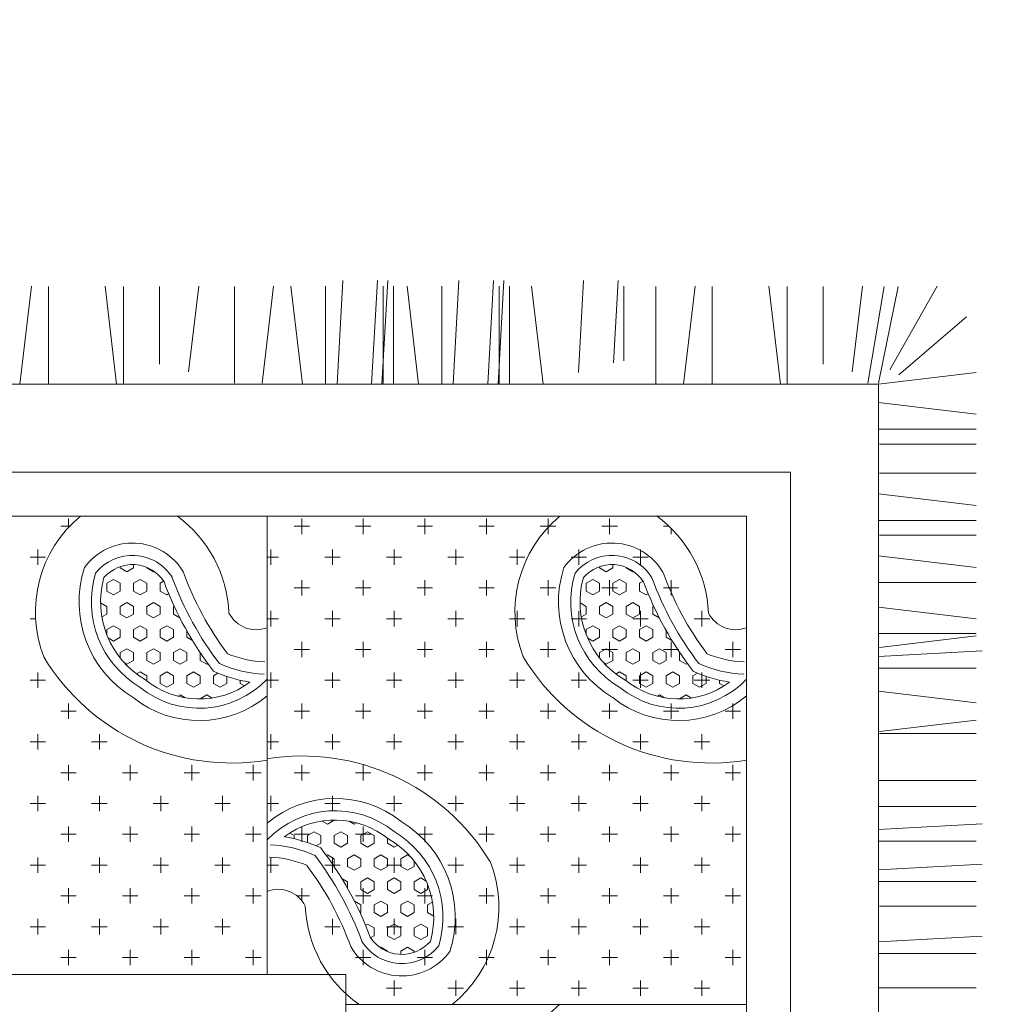
# Model space of a CAD drawing. Units: inches. Extents: x -638 to 186, y -762 to 59.
# Tile 10 of 31: x -117.58 to -100.41, y -474.18 to -456.78. Entities that reach past the tile are written whole.
import ezdxf

# ---------------------------------------------------------------- set-up
doc = ezdxf.new("R2010")
doc.units = ezdxf.units.IN
doc.layers.add('A-ANNO-DIMS', color=2, linetype='Continuous', lineweight=18)
doc.layers.add('furn', color=8, linetype='Continuous', lineweight=13)
doc.styles.get("Standard").update_dxf_attribs({"font": 'arial.ttf'})
doc.dimstyles.new('ISO-25', dxfattribs={"dimtxt": 4, "dimasz": 4, "dimexe": 1.25, "dimexo": 0.625, "dimtad": 0, "dimlunit": 4, "dimtxsty": 'Standard', "dimcen": 2.5, "dimclrt": 256, "dimadec": 0, "dimazin": 0, "dimtfac": 1, "dimtmove": 0, "dimatfit": 3, "dimfxl": 1, "dimfxlon": 1, "dimarcsym": 0})

# ---------------------------------------------------------------- blocks, each defined once
blk = doc.blocks.new('BED-DOUBLE-WITH-NIGHTSTANDS')
for p, q in [((58.548, 11.244), (58.548, 59.951)), ((68.982, 31.914), (68.982, 1.829)), ((67.427, 30.359), (67.427, 3.384)), ((66.65, 29.582), (66.65, 4.161)), ((68.982, 17.003), (70.71, 16.797)), ((59.394, 16.552), (59.394, 16.825)), ((60.483, 16.552), (60.483, 16.825)), ((61.571, 16.552), (61.571, 16.825)), ((62.659, 16.552), (62.659, 16.825)), ((63.748, 16.552), (63.748, 16.825)), ((64.836, 16.726), (64.836, 16.825)), ((65.924, 16.552), (65.924, 16.825)), ((59.258, 16.688), (59.53, 16.688)), ((60.346, 16.688), (60.619, 16.688)), ((61.435, 16.688), (61.707, 16.688)), ((62.523, 16.688), (62.795, 16.688)), ((63.612, 16.688), (63.884, 16.688)), ((65.788, 16.688), (66.06, 16.688)), ((68.982, 16.497), (70.707, 16.497)), ((58.85, 16.008), (58.85, 16.28)), ((59.938, 16.008), (59.938, 16.28)), ((61.027, 16.008), (61.027, 16.28)), ((62.115, 16.008), (62.115, 16.28)), ((63.203, 16.008), (63.203, 16.28)), ((66.468, 16.127), (66.468, 16.28)), ((58.714, 16.144), (58.986, 16.144)), ((59.802, 16.144), (60.074, 16.144)), ((60.891, 16.144), (61.163, 16.144)), ((61.979, 16.144), (62.251, 16.144)), ((63.067, 16.144), (63.339, 16.144)), ((66.45, 16.144), (66.605, 16.144)), ((59.394, 15.464), (59.394, 15.736)), ((60.483, 15.464), (60.483, 15.736)), ((61.571, 15.464), (61.571, 15.736)), ((62.659, 15.464), (62.659, 15.736)), ((59.258, 15.6), (59.53, 15.6)), ((60.346, 15.6), (60.619, 15.6)), ((61.435, 15.6), (61.707, 15.6)), ((62.523, 15.6), (62.795, 15.6)), ((64.917, 15.469), (64.866, 15.556)), ((65.053, 15.469), (65.116, 15.579)), ((68.982, 15.294), (70.71, 15.497)), ((64.44, 15.351), (64.495, 15.445)), ((64.508, 15.233), (64.44, 15.351)), ((64.552, 15.469), (64.644, 15.469)), ((64.712, 15.351), (64.644, 15.469)), ((64.644, 15.233), (64.712, 15.351)), ((64.917, 15.469), (65.053, 15.469)), ((65.257, 15.351), (65.325, 15.469)), ((65.325, 15.233), (65.257, 15.351)), ((65.325, 15.469), (65.461, 15.469)), ((65.529, 15.351), (65.461, 15.469)), ((65.461, 15.233), (65.529, 15.351)), ((58.85, 14.92), (58.85, 15.192)), ((59.938, 14.92), (59.938, 15.192)), ((61.027, 14.92), (61.027, 15.192)), ((62.115, 14.92), (62.115, 15.192)), ((64.032, 15.115), (64.059, 15.161)), ((64.143, 15.233), (64.236, 15.233)), ((64.304, 15.115), (64.236, 15.233)), ((64.508, 15.233), (64.644, 15.233)), ((64.849, 15.115), (64.917, 15.233)), ((64.917, 15.233), (65.053, 15.233)), ((65.121, 15.115), (65.053, 15.233)), ((65.325, 15.233), (65.461, 15.233)), ((65.665, 15.115), (65.733, 15.233)), ((65.733, 15.233), (65.755, 15.233)), ((68.982, 15.174), (70.707, 15.174)), ((58.714, 15.056), (58.986, 15.056)), ((59.802, 15.056), (60.074, 15.056)), ((60.891, 15.056), (61.163, 15.056)), ((61.979, 15.056), (62.251, 15.056)), ((64.1, 14.997), (64.032, 15.115)), ((64.1, 14.997), (64.236, 14.997)), ((64.236, 14.997), (64.304, 15.115)), ((64.44, 14.88), (64.508, 14.997)), ((64.508, 14.997), (64.644, 14.997)), ((64.712, 14.88), (64.644, 14.997)), ((64.917, 14.997), (64.849, 15.115)), ((64.917, 14.997), (65.053, 14.997)), ((65.053, 14.997), (65.121, 15.115)), ((65.257, 14.88), (65.325, 14.997)), ((65.325, 14.997), (65.461, 14.997)), ((65.529, 14.88), (65.461, 14.997)), ((65.733, 14.997), (65.665, 15.115)), ((65.733, 14.997), (65.791, 14.997)), ((63.828, 14.762), (63.896, 14.88)), ((63.896, 14.88), (63.86, 14.942)), ((64.508, 14.762), (64.44, 14.88)), ((64.644, 14.762), (64.712, 14.88)), ((65.325, 14.762), (65.257, 14.88)), ((65.461, 14.762), (65.529, 14.88)), ((59.394, 14.376), (59.394, 14.648)), ((60.483, 14.376), (60.483, 14.648)), ((61.571, 14.376), (61.571, 14.648)), ((63.737, 14.762), (63.828, 14.762)), ((64.032, 14.644), (64.1, 14.762)), ((64.1, 14.526), (64.032, 14.644)), ((64.1, 14.762), (64.236, 14.762)), ((64.304, 14.644), (64.236, 14.762)), ((64.236, 14.526), (64.304, 14.644)), ((64.508, 14.762), (64.644, 14.762)), ((64.849, 14.644), (64.917, 14.762)), ((64.917, 14.526), (64.849, 14.644)), ((64.917, 14.762), (65.053, 14.762)), ((65.121, 14.644), (65.053, 14.762)), ((65.053, 14.526), (65.121, 14.644)), ((65.325, 14.762), (65.461, 14.762)), ((65.665, 14.644), (65.733, 14.762)), ((65.671, 14.634), (65.665, 14.644)), ((65.733, 14.762), (65.741, 14.762)), ((59.258, 14.512), (59.53, 14.512)), ((60.346, 14.512), (60.619, 14.512)), ((61.435, 14.512), (61.707, 14.512)), ((63.624, 14.408), (63.692, 14.526)), ((63.692, 14.526), (63.828, 14.526)), ((63.896, 14.408), (63.828, 14.526)), ((64.1, 14.526), (64.236, 14.526)), ((64.44, 14.408), (64.508, 14.526)), ((64.508, 14.526), (64.644, 14.526)), ((64.712, 14.408), (64.644, 14.526)), ((64.917, 14.526), (65.053, 14.526)), ((65.257, 14.408), (65.325, 14.526)), ((65.325, 14.526), (65.461, 14.526)), ((65.497, 14.464), (65.461, 14.526)), ((69.331, 14.538), (70.707, 14.538)), ((63.692, 14.291), (63.624, 14.408)), ((63.692, 14.291), (63.828, 14.291)), ((63.828, 14.291), (63.896, 14.408)), ((64.032, 14.173), (64.1, 14.291)), ((64.1, 14.291), (64.236, 14.291)), ((64.304, 14.173), (64.236, 14.291)), ((64.508, 14.291), (64.44, 14.408)), ((64.508, 14.291), (64.644, 14.291)), ((64.644, 14.291), (64.712, 14.408)), ((64.852, 14.179), (64.917, 14.291)), ((64.917, 14.291), (65.053, 14.291)), ((65.059, 14.28), (65.053, 14.291)), ((65.276, 14.375), (65.257, 14.408)), ((58.85, 13.832), (58.85, 14.104)), ((59.938, 13.832), (59.938, 14.104)), ((61.027, 13.832), (61.027, 14.104)), ((62.115, 13.832), (62.115, 14.104)), ((63.438, 14.086), (63.488, 14.173)), ((63.488, 14.173), (63.465, 14.213)), ((64.1, 14.055), (64.032, 14.173)), ((64.236, 14.055), (64.304, 14.173)), ((58.714, 13.968), (58.986, 13.968)), ((59.802, 13.968), (60.074, 13.968)), ((60.891, 13.968), (61.163, 13.968)), ((61.979, 13.968), (62.251, 13.968)), ((63.624, 13.937), (63.692, 14.055)), ((63.692, 13.819), (63.624, 13.937)), ((63.692, 14.055), (63.828, 14.055)), ((63.896, 13.937), (63.828, 14.055)), ((63.828, 13.819), (63.896, 13.937)), ((64.1, 14.055), (64.236, 14.055)), ((64.451, 13.955), (64.508, 14.055)), ((64.508, 14.055), (64.621, 14.055)), ((69.195, 14.023), (70.71, 13.844)), ((63.417, 13.819), (63.42, 13.819)), ((63.488, 13.701), (63.42, 13.819)), ((63.692, 13.819), (63.828, 13.819)), ((64.032, 13.701), (64.1, 13.819)), ((64.1, 13.819), (64.236, 13.819)), ((64.237, 13.818), (64.236, 13.819)), ((63.434, 13.608), (63.488, 13.701)), ((63.624, 13.466), (63.692, 13.584)), ((63.692, 13.584), (63.828, 13.584)), ((63.874, 13.504), (63.828, 13.584)), ((64.043, 13.682), (64.032, 13.701)), ((59.258, 13.423), (59.53, 13.423)), ((59.394, 13.287), (59.394, 13.559)), ((60.346, 13.423), (60.619, 13.423)), ((60.483, 13.287), (60.483, 13.559)), ((61.435, 13.423), (61.707, 13.423)), ((61.571, 13.287), (61.571, 13.559)), ((63.692, 13.348), (63.624, 13.466)), ((63.692, 13.348), (63.815, 13.348)), ((63.648, 13.036), (63.692, 13.112)), ((63.692, 13.112), (63.748, 13.112)), ((68.996, 13.214), (70.707, 13.214)), ((58.714, 12.879), (58.986, 12.879)), ((58.85, 12.743), (58.85, 13.015)), ((59.802, 12.879), (60.074, 12.879)), ((59.938, 12.743), (59.938, 13.015)), ((60.891, 12.879), (61.163, 12.879)), ((61.027, 12.743), (61.027, 13.015)), ((61.979, 12.879), (62.251, 12.879)), ((62.115, 12.743), (62.115, 13.015)), ((68.996, 12.723), (70.71, 12.52)), ((66.65, 12.635), (58.548, 12.635)), ((58.548, 12.635), (66.65, 12.635)), ((60.346, 12.568), (60.619, 12.568)), ((60.483, 12.432), (60.483, 12.635)), ((61.435, 12.568), (61.707, 12.568)), ((61.571, 12.432), (61.571, 12.635)), ((62.523, 12.568), (62.795, 12.568)), ((62.523, 12.568), (62.795, 12.568)), ((62.659, 12.432), (62.659, 12.635)), ((62.659, 12.432), (62.659, 12.635)), ((63.612, 12.568), (63.884, 12.568)), ((63.612, 12.568), (63.884, 12.568)), ((63.748, 12.432), (63.748, 12.635)), ((63.748, 12.432), (63.748, 12.635)), ((64.7, 12.568), (64.972, 12.568)), ((64.7, 12.568), (64.972, 12.568)), ((64.836, 12.432), (64.836, 12.635)), ((64.836, 12.432), (64.836, 12.635)), ((65.788, 12.568), (66.06, 12.568)), ((65.788, 12.568), (66.06, 12.568)), ((65.924, 12.432), (65.924, 12.635)), ((65.924, 12.432), (65.924, 12.635)), ((66.65, 12.635), (66.65, 4.161)), ((61.047, 12.233), (61.003, 12.157)), ((68.982, 12.011), (70.71, 12.214)), ((59.857, 12.024), (60.074, 12.024)), ((59.938, 11.888), (59.938, 12.107)), ((60.891, 12.024), (61.163, 12.024)), ((61.003, 12.157), (60.948, 12.157)), ((61.027, 11.888), (61.027, 12.16)), ((61.979, 12.024), (62.251, 12.024)), ((62.115, 11.888), (62.115, 12.16)), ((63.067, 12.024), (63.339, 12.024)), ((63.067, 12.024), (63.339, 12.024)), ((63.203, 11.888), (63.203, 12.16)), ((63.203, 11.888), (63.203, 12.16)), ((64.156, 12.024), (64.428, 12.024)), ((64.156, 12.024), (64.428, 12.024)), ((64.292, 11.888), (64.292, 12.16)), ((64.292, 11.888), (64.292, 12.16)), ((65.244, 12.024), (65.516, 12.024)), ((65.244, 12.024), (65.516, 12.024)), ((65.38, 11.888), (65.38, 12.16)), ((65.38, 11.888), (65.38, 12.16)), ((66.332, 12.024), (66.605, 12.024)), ((66.332, 12.024), (66.605, 12.024)), ((66.468, 11.888), (66.468, 12.16)), ((66.468, 11.888), (66.468, 12.16)), ((61.003, 11.921), (60.881, 11.921)), ((61.003, 11.921), (61.072, 11.804)), ((60.821, 11.766), (60.867, 11.686)), ((61.003, 11.686), (60.867, 11.686)), ((61.072, 11.804), (61.003, 11.686)), ((61.261, 11.661), (61.208, 11.568)), ((59.394, 11.344), (59.394, 11.616)), ((60.483, 11.344), (60.483, 11.616)), ((60.663, 11.568), (60.595, 11.45)), ((60.652, 11.587), (60.663, 11.568)), ((61.208, 11.568), (61.276, 11.45)), ((61.571, 11.344), (61.571, 11.616)), ((62.659, 11.344), (62.659, 11.616)), ((62.659, 11.344), (62.659, 11.616)), ((63.748, 11.344), (63.748, 11.616)), ((63.748, 11.344), (63.748, 11.616)), ((64.836, 11.344), (64.836, 11.616)), ((64.836, 11.344), (64.836, 11.616)), ((65.924, 11.344), (65.924, 11.616)), ((65.924, 11.344), (65.924, 11.616)), ((68.982, 11.603), (70.71, 11.603)), ((59.258, 11.48), (59.53, 11.48)), ((60.245, 11.315), (60.187, 11.215)), ((60.346, 11.48), (60.619, 11.48)), ((60.459, 11.451), (60.459, 11.45)), ((60.595, 11.45), (60.459, 11.45)), ((60.867, 11.45), (60.799, 11.332)), ((60.799, 11.332), (60.867, 11.215)), ((61.003, 11.45), (60.867, 11.45)), ((61.003, 11.45), (61.072, 11.332)), ((61.072, 11.332), (61.003, 11.215)), ((61.279, 11.45), (61.276, 11.45)), ((61.435, 11.48), (61.707, 11.48)), ((62.523, 11.48), (62.795, 11.48)), ((62.523, 11.48), (62.795, 11.48)), ((63.612, 11.48), (63.884, 11.48)), ((63.612, 11.48), (63.884, 11.48)), ((64.7, 11.48), (64.972, 11.48)), ((64.7, 11.48), (64.972, 11.48)), ((65.788, 11.48), (66.06, 11.48)), ((65.788, 11.48), (66.06, 11.48)), ((68.982, 11.4), (70.811, 11.298)), ((20.158, 11.244), (58.548, 11.244)), ((58.022, 4.161), (58.022, 11.244)), ((58.022, 11.244), (58.022, 4.161)), ((60.187, 11.215), (60.075, 11.215)), ((60.459, 11.215), (60.391, 11.097)), ((60.595, 11.215), (60.459, 11.215)), ((60.595, 11.215), (60.663, 11.097)), ((61.003, 11.215), (60.867, 11.215)), ((61.258, 11.184), (61.208, 11.097)), ((58.85, 10.8), (58.85, 11.072)), ((59.637, 10.99), (59.643, 10.979)), ((59.779, 10.979), (59.643, 10.979)), ((59.843, 11.09), (59.779, 10.979)), ((59.938, 10.8), (59.938, 11.072)), ((60.051, 10.979), (59.983, 10.861)), ((60.187, 10.979), (60.051, 10.979)), ((60.187, 10.979), (60.255, 10.861)), ((60.391, 11.097), (60.459, 10.979)), ((60.595, 10.979), (60.459, 10.979)), ((60.663, 11.097), (60.595, 10.979)), ((60.867, 10.979), (60.799, 10.861)), ((61.003, 10.979), (60.867, 10.979)), ((61.003, 10.979), (61.072, 10.861)), ((61.027, 10.8), (61.027, 11.072)), ((61.208, 11.097), (61.231, 11.057)), ((62.115, 10.8), (62.115, 11.072)), ((63.203, 10.8), (63.203, 11.072)), ((63.203, 10.8), (63.203, 11.072)), ((64.292, 10.8), (64.292, 11.072)), ((64.292, 10.8), (64.292, 11.072)), ((65.38, 10.8), (65.38, 11.072)), ((65.38, 10.8), (65.38, 11.072)), ((66.468, 10.8), (66.468, 11.072)), ((66.468, 10.8), (66.468, 11.072)), ((58.714, 10.936), (58.986, 10.936)), ((59.199, 10.806), (59.235, 10.743)), ((59.439, 10.861), (59.371, 10.743)), ((59.419, 10.895), (59.439, 10.861)), ((59.802, 10.936), (60.074, 10.936)), ((59.983, 10.861), (60.051, 10.743)), ((60.255, 10.861), (60.187, 10.743)), ((60.799, 10.861), (60.867, 10.743)), ((60.891, 10.936), (61.163, 10.936)), ((61.072, 10.861), (61.003, 10.743)), ((61.979, 10.936), (62.251, 10.936)), ((63.067, 10.936), (63.339, 10.936)), ((63.067, 10.936), (63.339, 10.936)), ((64.156, 10.936), (64.428, 10.936)), ((64.156, 10.936), (64.428, 10.936)), ((65.244, 10.936), (65.516, 10.936)), ((65.244, 10.936), (65.516, 10.936)), ((66.332, 10.936), (66.605, 10.936)), ((66.332, 10.936), (66.605, 10.936)), ((68.982, 10.789), (70.811, 10.687)), ((59.031, 10.625), (58.963, 10.508)), ((59.025, 10.636), (59.031, 10.625)), ((59.371, 10.743), (59.235, 10.743)), ((59.643, 10.743), (59.575, 10.625)), ((59.575, 10.625), (59.643, 10.508)), ((59.779, 10.743), (59.643, 10.743)), ((59.779, 10.743), (59.847, 10.625)), ((59.847, 10.625), (59.779, 10.508)), ((60.187, 10.743), (60.051, 10.743)), ((60.459, 10.743), (60.391, 10.625)), ((60.391, 10.625), (60.459, 10.508)), ((60.595, 10.743), (60.459, 10.743)), ((60.595, 10.743), (60.663, 10.625)), ((60.663, 10.625), (60.595, 10.508)), ((61.003, 10.743), (60.867, 10.743)), ((58.306, 10.256), (58.306, 10.528)), ((58.963, 10.508), (58.955, 10.508)), ((59.235, 10.508), (59.167, 10.39)), ((59.371, 10.508), (59.235, 10.508)), ((59.371, 10.508), (59.439, 10.39)), ((59.394, 10.256), (59.394, 10.528)), ((59.779, 10.508), (59.643, 10.508)), ((60.051, 10.508), (59.983, 10.39)), ((60.187, 10.508), (60.051, 10.508)), ((60.187, 10.508), (60.255, 10.39)), ((60.595, 10.508), (60.459, 10.508)), ((60.483, 10.256), (60.483, 10.528)), ((60.867, 10.508), (60.799, 10.39)), ((60.958, 10.508), (60.867, 10.508)), ((61.571, 10.256), (61.571, 10.528)), ((62.659, 10.256), (62.659, 10.528)), ((62.659, 10.256), (62.659, 10.528)), ((63.748, 10.256), (63.748, 10.528)), ((63.748, 10.256), (63.748, 10.528)), ((64.836, 10.256), (64.836, 10.528)), ((64.836, 10.256), (64.836, 10.528)), ((65.924, 10.256), (65.924, 10.528)), ((65.924, 10.256), (65.924, 10.528)), ((68.982, 10.606), (70.811, 10.504)), ((68.982, 10.585), (70.71, 10.585)), ((58.17, 10.392), (58.442, 10.392)), ((58.963, 10.272), (58.904, 10.272)), ((58.963, 10.272), (59.031, 10.154)), ((59.167, 10.39), (59.235, 10.272)), ((59.371, 10.272), (59.235, 10.272)), ((59.258, 10.392), (59.53, 10.392)), ((59.439, 10.39), (59.371, 10.272)), ((59.643, 10.272), (59.575, 10.154)), ((59.779, 10.272), (59.643, 10.272)), ((59.779, 10.272), (59.847, 10.154)), ((59.983, 10.39), (60.051, 10.272)), ((60.187, 10.272), (60.051, 10.272)), ((60.255, 10.39), (60.187, 10.272)), ((60.346, 10.392), (60.619, 10.392)), ((60.459, 10.272), (60.391, 10.154)), ((60.595, 10.272), (60.459, 10.272)), ((60.595, 10.272), (60.663, 10.154)), ((60.799, 10.39), (60.836, 10.327)), ((61.435, 10.392), (61.707, 10.392)), ((62.523, 10.392), (62.795, 10.392)), ((62.523, 10.392), (62.795, 10.392)), ((63.612, 10.392), (63.884, 10.392)), ((63.612, 10.392), (63.884, 10.392)), ((64.7, 10.392), (64.972, 10.392)), ((64.7, 10.392), (64.972, 10.392)), ((65.788, 10.392), (66.06, 10.392)), ((65.788, 10.392), (66.06, 10.392)), ((68.982, 10.402), (70.71, 10.402)), ((59.031, 10.154), (58.963, 10.036)), ((59.575, 10.154), (59.643, 10.036)), ((59.847, 10.154), (59.779, 10.036)), ((60.391, 10.154), (60.459, 10.036)), ((60.663, 10.154), (60.637, 10.108)), ((68.982, 9.957), (70.71, 10.161)), ((58.85, 9.711), (58.85, 9.983)), ((58.963, 10.036), (58.94, 10.036)), ((59.235, 10.036), (59.167, 9.919)), ((59.167, 9.919), (59.235, 9.801)), ((59.371, 10.036), (59.235, 10.036)), ((59.371, 10.036), (59.439, 9.919)), ((59.439, 9.919), (59.371, 9.801)), ((59.779, 10.036), (59.643, 10.036)), ((59.938, 9.711), (59.938, 9.983)), ((60.051, 10.036), (59.983, 9.919)), ((59.983, 9.919), (60.051, 9.801)), ((60.187, 10.036), (60.051, 10.036)), ((60.187, 10.036), (60.255, 9.919)), ((60.255, 9.919), (60.201, 9.825)), ((60.553, 10.036), (60.459, 10.036)), ((61.027, 9.711), (61.027, 9.983)), ((62.115, 9.711), (62.115, 9.983)), ((62.115, 9.711), (62.115, 9.983)), ((63.203, 9.711), (63.203, 9.983)), ((63.203, 9.711), (63.203, 9.983)), ((64.292, 9.711), (64.292, 9.983)), ((64.292, 9.711), (64.292, 9.983)), ((65.38, 9.711), (65.38, 9.983)), ((65.38, 9.711), (65.38, 9.983)), ((66.468, 9.711), (66.468, 9.983)), ((66.468, 9.711), (66.468, 9.983)), ((58.714, 9.847), (58.986, 9.847)), ((59.371, 9.801), (59.235, 9.801)), ((59.643, 9.801), (59.58, 9.691)), ((59.779, 9.801), (59.643, 9.801)), ((59.779, 9.801), (59.83, 9.713)), ((59.802, 9.847), (60.074, 9.847)), ((60.144, 9.801), (60.051, 9.801)), ((60.891, 9.847), (61.163, 9.847)), ((61.979, 9.847), (62.251, 9.847)), ((61.979, 9.847), (62.251, 9.847)), ((63.067, 9.847), (63.339, 9.847)), ((63.067, 9.847), (63.339, 9.847)), ((64.156, 9.847), (64.428, 9.847)), ((64.156, 9.847), (64.428, 9.847)), ((65.244, 9.847), (65.516, 9.847)), ((65.244, 9.847), (65.516, 9.847)), ((66.332, 9.847), (66.605, 9.847)), ((66.332, 9.847), (66.605, 9.847)), ((58.306, 9.167), (58.306, 9.439)), ((59.394, 9.167), (59.394, 9.439)), ((60.483, 9.167), (60.483, 9.439)), ((61.571, 9.167), (61.571, 9.439)), ((61.571, 9.167), (61.571, 9.439)), ((62.659, 9.167), (62.659, 9.439)), ((62.659, 9.167), (62.659, 9.439)), ((63.748, 9.167), (63.748, 9.439)), ((63.748, 9.167), (63.748, 9.439)), ((64.836, 9.167), (64.836, 9.439)), ((64.836, 9.167), (64.836, 9.439)), ((65.924, 9.167), (65.924, 9.439)), ((65.924, 9.167), (65.924, 9.439)), ((68.982, 9.55), (70.71, 9.55)), ((58.17, 9.303), (58.442, 9.303)), ((59.258, 9.303), (59.53, 9.303)), ((60.346, 9.303), (60.619, 9.303)), ((61.435, 9.303), (61.707, 9.303)), ((61.435, 9.303), (61.707, 9.303)), ((62.523, 9.303), (62.795, 9.303)), ((62.523, 9.303), (62.795, 9.303)), ((63.612, 9.303), (63.884, 9.303)), ((63.612, 9.303), (63.884, 9.303)), ((64.7, 9.303), (64.972, 9.303)), ((64.7, 9.303), (64.972, 9.303)), ((65.788, 9.303), (66.06, 9.303)), ((65.788, 9.303), (66.06, 9.303)), ((68.982, 9.347), (70.811, 9.245)), ((58.85, 8.623), (58.85, 8.895)), ((59.938, 8.623), (59.938, 8.895)), ((61.027, 8.623), (61.027, 8.895)), ((61.027, 8.623), (61.027, 8.895)), ((62.115, 8.623), (62.115, 8.895)), ((62.115, 8.623), (62.115, 8.895)), ((63.203, 8.623), (63.203, 8.895)), ((63.203, 8.623), (63.203, 8.895)), ((64.292, 8.623), (64.292, 8.895)), ((64.292, 8.623), (64.292, 8.895)), ((65.38, 8.623), (65.38, 8.895)), ((65.38, 8.623), (65.38, 8.895)), ((66.468, 8.623), (66.468, 8.895)), ((66.468, 8.623), (66.468, 8.895)), ((58.714, 8.759), (58.783, 8.759)), ((58.714, 8.759), (58.986, 8.759)), ((58.85, 8.623), (58.85, 8.728)), ((59.802, 8.759), (60.074, 8.759)), ((60.891, 8.759), (61.163, 8.759)), ((60.891, 8.759), (61.163, 8.759)), ((61.979, 8.759), (62.251, 8.759)), ((61.979, 8.759), (62.251, 8.759)), ((63.067, 8.759), (63.339, 8.759)), ((63.067, 8.759), (63.339, 8.759)), ((64.156, 8.759), (64.428, 8.759)), ((64.156, 8.759), (64.428, 8.759)), ((65.244, 8.759), (65.516, 8.759)), ((65.244, 8.759), (65.516, 8.759)), ((66.332, 8.759), (66.605, 8.759)), ((66.332, 8.759), (66.605, 8.759)), ((68.982, 8.736), (70.811, 8.634)), ((68.982, 8.553), (70.811, 8.451)), ((68.982, 8.532), (70.71, 8.532)), ((58.306, 8.079), (58.306, 8.351)), ((58.306, 8.079), (58.306, 8.351)), ((59.394, 8.079), (59.394, 8.351)), ((59.394, 8.079), (59.394, 8.351)), ((60.483, 8.079), (60.483, 8.351)), ((60.483, 8.079), (60.483, 8.351)), ((61.571, 8.079), (61.571, 8.351)), ((61.571, 8.079), (61.571, 8.351)), ((62.659, 8.079), (62.659, 8.351)), ((62.659, 8.079), (62.659, 8.351)), ((63.748, 8.079), (63.748, 8.351)), ((63.748, 8.079), (63.748, 8.351)), ((64.836, 8.253), (64.836, 8.351)), ((64.836, 8.079), (64.836, 8.351)), ((65.924, 8.079), (65.924, 8.351)), ((65.924, 8.079), (65.924, 8.351)), ((58.17, 8.215), (58.442, 8.215)), ((58.17, 8.215), (58.442, 8.215)), ((59.258, 8.215), (59.53, 8.215)), ((59.258, 8.215), (59.53, 8.215)), ((60.346, 8.215), (60.619, 8.215)), ((60.346, 8.215), (60.619, 8.215)), ((61.435, 8.215), (61.707, 8.215)), ((61.435, 8.215), (61.707, 8.215)), ((62.523, 8.215), (62.795, 8.215)), ((62.523, 8.215), (62.795, 8.215)), ((63.612, 8.215), (63.884, 8.215)), ((63.612, 8.215), (63.884, 8.215)), ((64.7, 8.215), (64.972, 8.215)), ((65.788, 8.215), (66.06, 8.215)), ((65.788, 8.215), (66.06, 8.215)), ((68.982, 8.349), (70.71, 8.349)), ((68.982, 7.757), (70.71, 7.961)), ((58.714, 7.671), (58.986, 7.671)), ((58.714, 7.671), (58.986, 7.671)), ((58.85, 7.535), (58.85, 7.807)), ((58.85, 7.535), (58.85, 7.807)), ((59.802, 7.671), (60.074, 7.671)), ((59.802, 7.671), (60.074, 7.671)), ((59.938, 7.535), (59.938, 7.807)), ((59.938, 7.535), (59.938, 7.807)), ((60.891, 7.671), (61.163, 7.671)), ((60.891, 7.671), (61.163, 7.671)), ((61.027, 7.535), (61.027, 7.807)), ((61.027, 7.535), (61.027, 7.807)), ((61.979, 7.671), (62.251, 7.671)), ((61.979, 7.671), (62.251, 7.671)), ((62.115, 7.535), (62.115, 7.807)), ((62.115, 7.535), (62.115, 7.807)), ((63.067, 7.671), (63.339, 7.671)), ((63.067, 7.671), (63.339, 7.671)), ((63.203, 7.535), (63.203, 7.807)), ((63.203, 7.535), (63.203, 7.807)), ((64.156, 7.671), (64.428, 7.671)), ((64.292, 7.535), (64.292, 7.807)), ((65.244, 7.671), (65.516, 7.671)), ((65.38, 7.535), (65.38, 7.807)), ((66.332, 7.671), (66.605, 7.671)), ((66.45, 7.671), (66.605, 7.671)), ((66.468, 7.653), (66.468, 7.807)), ((66.468, 7.535), (66.468, 7.807)), ((58.306, 6.99), (58.306, 7.263)), ((58.306, 6.99), (58.306, 7.263)), ((59.394, 6.99), (59.394, 7.263)), ((59.394, 6.99), (59.394, 7.263)), ((60.483, 6.99), (60.483, 7.263)), ((60.483, 6.99), (60.483, 7.263)), ((61.571, 6.99), (61.571, 7.263)), ((61.571, 6.99), (61.571, 7.263)), ((62.659, 6.99), (62.659, 7.263)), ((62.659, 6.99), (62.659, 7.263)), ((63.748, 6.99), (63.748, 7.263)), ((64.836, 6.99), (64.836, 7.263)), ((65.924, 6.99), (65.924, 7.263)), ((69.184, 7.135), (70.811, 7.044)), ((58.17, 7.127), (58.442, 7.127)), ((58.17, 7.127), (58.442, 7.127)), ((59.258, 7.127), (59.53, 7.127)), ((59.258, 7.127), (59.53, 7.127)), ((60.346, 7.127), (60.619, 7.127)), ((60.346, 7.127), (60.619, 7.127)), ((61.435, 7.127), (61.707, 7.127)), ((61.435, 7.127), (61.707, 7.127)), ((62.523, 7.127), (62.795, 7.127)), ((62.523, 7.127), (62.795, 7.127)), ((63.612, 7.127), (63.884, 7.127)), ((64.44, 6.877), (64.495, 6.971)), ((64.552, 6.995), (64.644, 6.995)), ((64.712, 6.877), (64.644, 6.995)), ((64.7, 7.127), (64.972, 7.127)), ((64.917, 6.995), (64.866, 7.082)), ((64.917, 6.995), (65.053, 6.995)), ((65.053, 6.995), (65.116, 7.105)), ((65.257, 6.877), (65.325, 6.995)), ((65.325, 6.995), (65.461, 6.995)), ((65.529, 6.877), (65.461, 6.995)), ((65.788, 7.127), (66.06, 7.127)), ((64.508, 6.76), (64.44, 6.877)), ((64.644, 6.76), (64.712, 6.877)), ((65.325, 6.76), (65.257, 6.877)), ((65.461, 6.76), (65.529, 6.877)), ((58.85, 6.446), (58.85, 6.718)), ((58.85, 6.446), (58.85, 6.718)), ((59.938, 6.446), (59.938, 6.718)), ((59.938, 6.446), (59.938, 6.718)), ((61.027, 6.446), (61.027, 6.718)), ((61.027, 6.446), (61.027, 6.718)), ((62.115, 6.446), (62.115, 6.718)), ((62.115, 6.446), (62.115, 6.718)), ((63.203, 6.446), (63.203, 6.718)), ((64.032, 6.642), (64.059, 6.688)), ((64.1, 6.524), (64.032, 6.642)), ((64.143, 6.76), (64.236, 6.76)), ((64.304, 6.642), (64.236, 6.76)), ((64.236, 6.524), (64.304, 6.642)), ((64.292, 6.446), (64.292, 6.718)), ((64.508, 6.76), (64.644, 6.76)), ((64.849, 6.642), (64.917, 6.76)), ((64.917, 6.524), (64.849, 6.642)), ((64.917, 6.76), (65.053, 6.76)), ((65.121, 6.642), (65.053, 6.76)), ((65.053, 6.524), (65.121, 6.642)), ((65.325, 6.76), (65.461, 6.76)), ((65.38, 6.446), (65.38, 6.718)), ((65.665, 6.642), (65.733, 6.76)), ((65.733, 6.524), (65.665, 6.642)), ((65.733, 6.76), (65.755, 6.76)), ((66.468, 6.446), (66.468, 6.718)), ((58.714, 6.582), (58.986, 6.582)), ((58.714, 6.582), (58.986, 6.582)), ((59.802, 6.582), (60.074, 6.582)), ((59.802, 6.582), (60.074, 6.582)), ((60.891, 6.582), (61.163, 6.582)), ((60.891, 6.582), (61.163, 6.582)), ((61.979, 6.582), (62.251, 6.582)), ((61.979, 6.582), (62.251, 6.582)), ((63.067, 6.582), (63.339, 6.582)), ((63.896, 6.406), (63.86, 6.469)), ((64.1, 6.524), (64.236, 6.524)), ((64.156, 6.582), (64.428, 6.582)), ((64.44, 6.406), (64.508, 6.524)), ((64.508, 6.524), (64.644, 6.524)), ((64.712, 6.406), (64.644, 6.524)), ((64.917, 6.524), (65.053, 6.524)), ((65.244, 6.582), (65.516, 6.582)), ((65.257, 6.406), (65.325, 6.524)), ((65.325, 6.524), (65.461, 6.524)), ((65.529, 6.406), (65.461, 6.524)), ((65.733, 6.524), (65.791, 6.524)), ((66.332, 6.582), (66.605, 6.582)), ((69.357, 6.514), (70.811, 6.433)), ((63.737, 6.288), (63.828, 6.288)), ((63.828, 6.288), (63.896, 6.406)), ((64.032, 6.17), (64.1, 6.288)), ((64.1, 6.288), (64.236, 6.288)), ((64.304, 6.17), (64.236, 6.288)), ((64.508, 6.288), (64.44, 6.406)), ((64.508, 6.288), (64.644, 6.288)), ((64.644, 6.288), (64.712, 6.406)), ((64.849, 6.17), (64.917, 6.288)), ((64.917, 6.288), (65.053, 6.288)), ((65.121, 6.17), (65.053, 6.288)), ((65.325, 6.288), (65.257, 6.406)), ((65.325, 6.288), (65.461, 6.288)), ((65.461, 6.288), (65.529, 6.406)), ((65.665, 6.17), (65.733, 6.288)), ((65.733, 6.288), (65.741, 6.288)), ((69.393, 6.332), (70.71, 6.332)), ((58.306, 5.902), (58.306, 6.174)), ((58.306, 5.902), (58.306, 6.174)), ((59.394, 5.902), (59.394, 6.174)), ((59.394, 5.902), (59.394, 6.174)), ((60.483, 5.902), (60.483, 6.174)), ((60.483, 5.902), (60.483, 6.174)), ((61.571, 5.902), (61.571, 6.174)), ((61.571, 5.902), (61.571, 6.174)), ((62.659, 5.902), (62.659, 6.174)), ((63.748, 5.902), (63.748, 6.174)), ((64.1, 6.053), (64.032, 6.17)), ((64.236, 6.053), (64.304, 6.17)), ((64.836, 5.902), (64.836, 6.174)), ((64.917, 6.053), (64.849, 6.17)), ((65.053, 6.053), (65.121, 6.17)), ((65.671, 6.16), (65.665, 6.17)), ((65.924, 5.902), (65.924, 6.174)), ((58.17, 6.038), (58.442, 6.038)), ((58.17, 6.038), (58.442, 6.038)), ((59.258, 6.038), (59.53, 6.038)), ((59.258, 6.038), (59.53, 6.038)), ((60.346, 6.038), (60.619, 6.038)), ((60.346, 6.038), (60.619, 6.038)), ((61.435, 6.038), (61.707, 6.038)), ((61.435, 6.038), (61.707, 6.038)), ((62.523, 6.038), (62.795, 6.038)), ((63.612, 6.038), (63.884, 6.038)), ((63.624, 5.935), (63.692, 6.053)), ((63.692, 5.817), (63.624, 5.935)), ((63.692, 6.053), (63.828, 6.053)), ((63.896, 5.935), (63.828, 6.053)), ((63.828, 5.817), (63.896, 5.935)), ((64.1, 6.053), (64.236, 6.053)), ((64.44, 5.935), (64.508, 6.053)), ((64.508, 5.817), (64.44, 5.935)), ((64.508, 6.053), (64.644, 6.053)), ((64.712, 5.935), (64.644, 6.053)), ((64.644, 5.817), (64.712, 5.935)), ((64.7, 6.038), (64.972, 6.038)), ((64.917, 6.053), (65.053, 6.053)), ((65.257, 5.935), (65.325, 6.053)), ((65.276, 5.901), (65.257, 5.935)), ((65.325, 6.053), (65.461, 6.053)), ((65.497, 5.99), (65.461, 6.053)), ((65.788, 6.038), (66.06, 6.038)), ((63.692, 5.817), (63.828, 5.817)), ((64.032, 5.699), (64.1, 5.817)), ((64.1, 5.817), (64.236, 5.817)), ((64.304, 5.699), (64.236, 5.817)), ((64.508, 5.817), (64.644, 5.817)), ((64.852, 5.706), (64.917, 5.817)), ((64.917, 5.817), (65.053, 5.817)), ((65.059, 5.806), (65.053, 5.817)), ((68.982, 5.764), (70.707, 5.764)), ((58.85, 5.358), (58.85, 5.63)), ((58.85, 5.358), (58.85, 5.63)), ((59.938, 5.358), (59.938, 5.63)), ((59.938, 5.358), (59.938, 5.63)), ((61.027, 5.358), (61.027, 5.63)), ((61.027, 5.358), (61.027, 5.63)), ((62.115, 5.358), (62.115, 5.63)), ((62.115, 5.358), (62.115, 5.63)), ((63.203, 5.358), (63.203, 5.63)), ((63.438, 5.612), (63.488, 5.699)), ((63.488, 5.699), (63.465, 5.739)), ((63.624, 5.464), (63.692, 5.581)), ((63.692, 5.581), (63.828, 5.581)), ((63.896, 5.464), (63.828, 5.581)), ((64.1, 5.581), (64.032, 5.699)), ((64.1, 5.581), (64.236, 5.581)), ((64.236, 5.581), (64.304, 5.699)), ((64.292, 5.358), (64.292, 5.63)), ((64.451, 5.481), (64.508, 5.581)), ((64.508, 5.581), (64.621, 5.581)), ((65.38, 5.358), (65.38, 5.63)), ((66.468, 5.533), (66.468, 5.63)), ((58.714, 5.494), (58.986, 5.494)), ((58.714, 5.494), (58.986, 5.494)), ((59.802, 5.494), (60.074, 5.494)), ((59.802, 5.494), (60.074, 5.494)), ((60.891, 5.494), (61.163, 5.494)), ((60.891, 5.494), (61.163, 5.494)), ((61.979, 5.494), (62.251, 5.494)), ((61.979, 5.494), (62.251, 5.494)), ((63.067, 5.494), (63.339, 5.494)), ((63.692, 5.346), (63.624, 5.464)), ((63.828, 5.346), (63.896, 5.464)), ((64.156, 5.494), (64.428, 5.494)), ((65.244, 5.494), (65.516, 5.494)), ((66.332, 5.494), (66.43, 5.494)), ((63.417, 5.346), (63.42, 5.346)), ((63.488, 5.228), (63.42, 5.346)), ((63.434, 5.135), (63.488, 5.228)), ((63.692, 5.346), (63.828, 5.346)), ((64.032, 5.228), (64.1, 5.346)), ((64.043, 5.209), (64.032, 5.228)), ((64.1, 5.346), (64.236, 5.346)), ((64.237, 5.344), (64.236, 5.346)), ((68.982, 5.274), (70.71, 5.069)), ((58.306, 4.814), (58.306, 5.086)), ((58.306, 4.814), (58.306, 5.086)), ((59.394, 4.814), (59.394, 5.086)), ((59.394, 4.814), (59.394, 5.086)), ((60.483, 4.814), (60.483, 5.086)), ((60.483, 4.814), (60.483, 5.086)), ((61.571, 4.814), (61.571, 5.086)), ((61.571, 4.814), (61.571, 5.086)), ((62.659, 4.814), (62.659, 5.086)), ((63.624, 4.992), (63.692, 5.11)), ((63.692, 5.11), (63.828, 5.11)), ((63.748, 4.814), (63.748, 5.086)), ((63.874, 5.03), (63.828, 5.11)), ((64.836, 4.814), (64.836, 5.086)), ((58.17, 4.95), (58.442, 4.95)), ((58.17, 4.95), (58.442, 4.95)), ((59.258, 4.95), (59.53, 4.95)), ((59.258, 4.95), (59.53, 4.95)), ((60.346, 4.95), (60.619, 4.95)), ((60.346, 4.95), (60.619, 4.95)), ((61.435, 4.95), (61.707, 4.95)), ((61.435, 4.95), (61.707, 4.95)), ((62.523, 4.95), (62.795, 4.95)), ((63.612, 4.95), (63.884, 4.95)), ((63.692, 4.874), (63.624, 4.992)), ((63.692, 4.874), (63.815, 4.874)), ((64.7, 4.95), (64.972, 4.95)), ((68.982, 4.769), (70.707, 4.769)), ((58.85, 4.27), (58.85, 4.542)), ((58.85, 4.27), (58.85, 4.542)), ((59.938, 4.27), (59.938, 4.542)), ((59.938, 4.27), (59.938, 4.542)), ((61.027, 4.27), (61.027, 4.542)), ((61.027, 4.27), (61.027, 4.542)), ((62.115, 4.27), (62.115, 4.542)), ((62.115, 4.27), (62.115, 4.542)), ((63.203, 4.27), (63.203, 4.542)), ((63.648, 4.563), (63.692, 4.639)), ((63.692, 4.639), (63.748, 4.639)), ((64.292, 4.27), (64.292, 4.542)), ((58.714, 4.406), (58.986, 4.406)), ((58.714, 4.406), (58.986, 4.406)), ((59.802, 4.406), (60.074, 4.406)), ((59.802, 4.406), (60.074, 4.406)), ((60.891, 4.406), (61.163, 4.406)), ((60.891, 4.406), (61.163, 4.406)), ((61.979, 4.406), (62.251, 4.406)), ((61.979, 4.406), (62.251, 4.406)), ((63.067, 4.406), (63.339, 4.406)), ((64.156, 4.406), (64.428, 4.406)), ((66.65, 4.161), (40.767, 4.161)), ((66.65, 4.161), (58.022, 4.161)), ((68.982, 3.565), (70.71, 3.769)), ((67.427, 3.384), (39.99, 3.384)), ((68.982, 3.446), (70.707, 3.446)), ((69.331, 2.81), (70.707, 2.81)), ((69.195, 2.295), (70.71, 2.115)), ((68.996, 2.022), (70.707, 1.732)), ((68.982, 1.829), (38.435, 1.829)), ((58.312, 1.829), (58.312, 0.102)), ((58.923, 1.829), (58.923, 0.102)), ((59.126, 1.829), (59.228, 0)), ((59.755, 1.815), (59.755, 0.105)), ((60.193, 1.829), (60.193, 0.102)), ((60.397, 1.829), (60.499, 0)), ((60.906, 1.829), (60.906, 0.102)), ((61.11, 1.829), (61.212, 0)), ((61.517, 1.829), (61.517, 0.102)), ((61.977, 1.829), (61.977, 0.102)), ((62.81, 1.815), (62.81, 0.105)), ((62.841, 1.815), (63.044, 0.102)), ((63.554, 1.829), (63.35, 0.102)), ((63.961, 1.829), (63.961, 0.102)), ((64.165, 1.829), (64.266, 0)), ((64.327, 1.815), (64.531, 0.102)), ((64.572, 1.829), (64.572, 0.102)), ((65.04, 1.829), (64.836, 0.102)), ((65.476, 1.829), (65.476, 0.102)), ((65.944, 1.829), (65.741, 0.102)), ((66.309, 1.815), (66.309, 0.105)), ((66.573, 1.829), (66.573, 0.102)), ((67.041, 1.829), (66.838, 0.102)), ((67.406, 1.815), (67.406, 0.105)), ((67.922, 1.815), (67.922, 0.105)), ((68.186, 1.829), (68.186, 0.102)), ((68.654, 1.829), (68.45, 0.102)), ((68.982, 1.829), (69.186, 0.102)), ((68.996, 1.829), (70.707, 1.486)), ((69.232, 1.631), (70.71, 0.792)), ((69.142, 1.47), (70.169, 0.275))]:
    blk.add_line(p, q)
for centre, radius, start, end in [((64.955, 14.528), 2.202, 39.6653, 111.1583), ((66.165, 13.26), 3.88, 121.1125, 189.2666), ((65.133, 13.987), 1.972, 72.055, 149.019), ((65.126, 15.016), 1.047, 300.344, 54.0192), ((65.133, 13.987), 1.754, 73.2189, 149.4808), ((65.126, 15.016), 0.829, 301.6232, 51.6957), ((65.133, 13.987), 1.591, 74.3738, 149.9117), ((65.126, 15.016), 0.666, 302.9498, 49.099), ((64.914, 13.836), 1.878, 141.5973, 219.7611), ((64.914, 13.836), 1.66, 141.1107, 226.3387), ((64.914, 13.836), 1.497, 140.6541, 216.833), ((67.553, 8.875), 5.952, 110.2997, 127.7385), ((67.553, 8.875), 5.789, 110.1318, 127.346), ((67.553, 8.875), 5.571, 109.9219, 126.7677), ((64.84, 15.553), 2.246, 272.4675, 323.7193), ((65.96, 12.613), 2.268, 154.7059, 171.7535), ((65.96, 12.613), 2.104, 155.7609, 178.0373), ((65.96, 12.613), 1.887, 157.4091, 178.0373), ((65.181, 12.828), 0.54, 117.0088, 201.0409), ((59.514, 12.441), 0.54, 297.0088, 21.0409), ((58.736, 12.656), 1.887, 337.4091, 358.0373), ((58.53, 12.01), 3.88, 301.1125, 9.2666), ((58.736, 12.656), 2.104, 335.7609, 358.0373), ((59.782, 11.434), 1.66, 321.1107, 46.3387), ((59.782, 11.434), 1.878, 321.5973, 39.7611), ((58.736, 12.656), 2.268, 334.7059, 351.7535), ((59.782, 11.434), 1.497, 320.6541, 36.833), ((59.856, 9.717), 2.246, 92.4675, 144.7393), ((57.143, 16.395), 5.571, 289.9219, 306.7677), ((57.143, 16.395), 5.789, 290.1318, 307.346), ((57.143, 16.395), 5.952, 290.2997, 307.7385), ((59.57, 10.253), 1.047, 120.344, 234.0192), ((59.57, 10.253), 0.829, 121.6232, 231.6957), ((59.57, 10.253), 0.666, 122.9498, 229.099), ((59.563, 11.282), 1.591, 254.3738, 329.9117), ((59.563, 11.282), 1.972, 252.055, 329.019), ((59.563, 11.282), 1.754, 253.2189, 329.4808), ((59.74, 10.742), 2.202, 218.7027, 291.1583), ((56.328, 6.054), 2.202, 39.6653, 111.1583), ((64.955, 6.054), 2.202, 39.6653, 111.1583), ((66.165, 4.786), 3.88, 121.1125, 189.2666), ((65.133, 5.514), 1.972, 72.055, 149.019), ((65.126, 6.543), 1.047, 300.344, 54.0192), ((65.133, 5.514), 1.754, 73.2189, 149.4808), ((65.126, 6.543), 0.829, 301.6232, 51.6957), ((65.133, 5.514), 1.591, 74.3738, 149.9117), ((65.126, 6.543), 0.666, 302.9498, 49.099), ((64.914, 5.362), 1.878, 141.5973, 219.7611), ((64.914, 5.362), 1.66, 141.1107, 226.3387), ((64.914, 5.362), 1.497, 140.6541, 216.833), ((67.553, 0.401), 5.952, 110.2997, 127.7385), ((67.553, 0.401), 5.789, 110.1318, 127.346), ((64.84, 7.079), 2.246, 272.4675, 323.7193), ((67.553, 0.401), 5.571, 109.9219, 126.7677), ((65.96, 4.14), 2.268, 154.7059, 171.7535), ((65.96, 4.14), 2.104, 155.7609, 178.0373), ((65.96, 4.14), 1.887, 157.4091, 178.0373), ((65.181, 4.355), 0.54, 117.0088, 201.0409)]:
    blk.add_arc(centre, radius, start, end)
blk = doc.blocks.new('*D38')
at = {"layer": 'A-ANNO-DIMS', "color": 0, "lineweight": -2, "transparency": 16777216}
for p, q in [((182.663, -280.533), (184.913, -280.533)), ((183.663, -284.533), (183.663, -371.726)), ((183.663, -473.533), (183.663, -386.34)), ((182.663, -477.533), (184.913, -477.533))]:
    blk.add_line(p, q, dxfattribs=at)
at = {"layer": 'A-ANNO-DIMS', "color": 0, "lineweight": 30, "transparency": 16777216}
for points in [[(182.997, -284.533), (184.33, -284.533), (183.663, -280.533)], [(182.997, -473.533), (184.33, -473.533), (183.663, -477.533)]]:
    blk.add_solid(points, dxfattribs=at)
at = {"layer": 'Defpoints', "color": 0, "lineweight": 30, "transparency": 16777216}
for p in [(-404.526, -280.533), (-404.526, -477.533), (183.663, -477.533)]:
    blk.add_point(p, dxfattribs=at)
at = {"layer": 'A-ANNO-DIMS', "transparency": 16777216, "insert": (183.663, -379.033), "char_height": 4, "attachment_point": 5, "rotation": 90}
blk.add_mtext('16\'-5"', dxfattribs=at)

msp = doc.modelspace()

# ---------------------------------------------------------------- block references
at = {"layer": 'furn', "rotation": 90.00000000000017}
msp.add_blockref('BED-DOUBLE-WITH-NIGHTSTANDS', (-100.575, -532.203), dxfattribs=at)

# ---------------------------------------------------------------- dimensions: what is measured, and where the dimension line sits
at = {"layer": 'A-ANNO-DIMS'}
dim = msp.add_linear_dim(base=(183.663, -477.533), p1=(-404.526, -280.533), p2=(-404.526, -477.533), angle=90, dimstyle='ISO-25', override={"dimdec": 1, "dimlfac": 1, "dimrnd": 0, "dimzin": 1, "dimdsep": 46, "dimlunit": 4, "dimfrac": 2}, dxfattribs=at)
dim.commit()
dim.dimension.update_dxf_attribs({"geometry": '*D38', "text_midpoint": (183.663, -379.033)})

doc.saveas('drawing.dxf')
